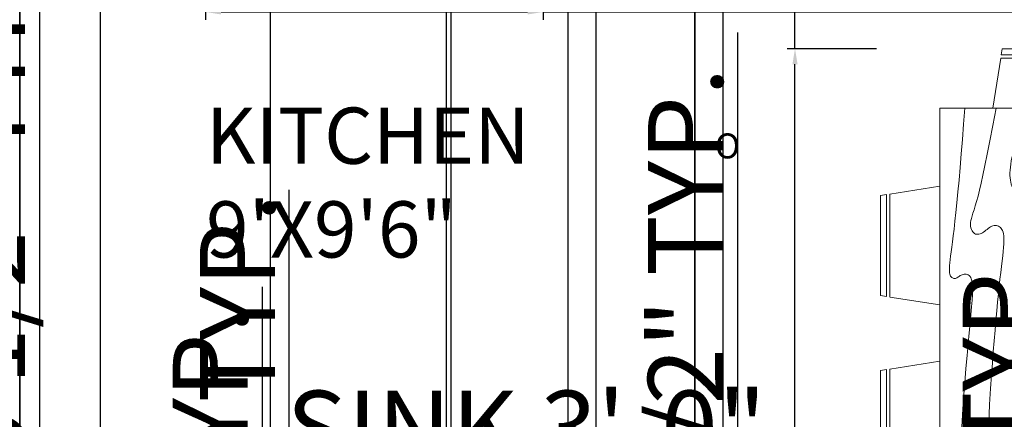
# Model space of a CAD drawing. Units: inches. Extents: x 2691 to 3133, y 1294 to 1993.
# Tile 5 of 7: x 2777 to 2935, y 1798 to 1862. Entities that reach past the tile are written whole.
import ezdxf

# ---------------------------------------------------------------- set-up
doc = ezdxf.new("R2010")
doc.units = ezdxf.units.IN
for name, color, linetype, lineweight in [('A-ANNO-DIMS', 2, 'Continuous', 18), ('A-ANNO-TEXT', 7, 'Continuous', 18), ('A-AREA-IDEN', 7, 'Continuous', 25), ('A-FURN', 8, 'Continuous', 18), ('A-WALL', 7, 'Continuous', 35)]:
    doc.layers.add(name, color=color, linetype=linetype, lineweight=lineweight)
doc.styles.get("Standard").update_dxf_attribs({"font": 'arial.ttf'})
doc.dimstyles.new('ISO-25', dxfattribs={"dimtxt": 12, "dimasz": 2.5, "dimexe": 1.25, "dimexo": 0.625, "dimtad": 1, "dimdec": 1, "dimlunit": 3, "dimtxsty": 'Standard', "dimcen": 2.5, "dimadec": 0, "dimazin": 0, "dimtfac": 1, "dimtdec": 1, "dimtmove": 0, "dimatfit": 3, "dimfxl": 1, "dimarcsym": 0})

# ---------------------------------------------------------------- blocks, each defined once
blk = doc.blocks.new('Dining Set - 36 x 72 in.')
for p, q in [((-22, 27.5), (-22.1562, 26.50042)), ((-22, 27.5), (-6, 27.5)), ((-5.8437, 26.49966), (-6, 27.5)), ((6, 27.5), (5.8438, 26.50042)), ((6, 27.5), (22, 27.5)), ((22.1563, 26.49966), (22, 27.5)), ((-22.2343, 26.00059), (-23.4847, 17.99762)), ((-22.2304, 26), (-5.7608, 26)), ((-5.8416, 26.5), (-22.1534, 26.5)), ((-4.5152, 17.99762), (-5.7655, 25.99926)), ((5.7657, 26.00059), (4.5153, 17.99762)), ((5.7696, 26), (22.2392, 26)), ((22.1584, 26.5), (5.8466, 26.5)), ((23.4848, 17.99762), (22.2345, 25.99926)), ((36, 18), (-36, 18)), ((-36, 18), (-36, -18)), ((36, -18), (36, 18)), ((-44.0006, 8.23428), (-35.9976, 9.48474)), ((44.0006, 8.23428), (35.9976, 9.48474)), ((-45.5, 8), (-44.5004, 8.15617)), ((-45.5, 8), (-45.5, -8)), ((-44.5, -8.15843), (-44.5, 8.15338)), ((-44, 8.23041), (-44, -8.23915)), ((44, 8.23041), (44, -8.23915)), ((44.5, -8.15843), (44.5, 8.15338)), ((45.5, 8), (44.5005, 8.15617)), ((45.5, 8), (45.5, -8)), ((-44.4997, -8.15631), (-45.5, -8)), ((-35.9976, -9.48476), (-43.9993, -8.2345)), ((35.9976, -9.48476), (43.9993, -8.2345)), ((44.4997, -8.15631), (45.5, -8)), ((-36, -18), (36, -18)), ((-22.2343, -26.0006), (-23.4847, -17.99762)), ((-4.5152, -17.99762), (-5.7655, -25.99928)), ((5.7657, -26.0006), (4.5153, -17.99762)), ((23.4848, -17.99762), (22.2345, -25.99928)), ((-22.2304, -26), (-5.7608, -26)), ((-22, -27.5), (-22.1562, -26.50044)), ((-5.8416, -26.5), (-22.1534, -26.5)), ((-5.8437, -26.49967), (-6, -27.5)), ((5.7696, -26), (22.2392, -26)), ((6, -27.5), (5.8438, -26.50044)), ((22.1584, -26.5), (5.8466, -26.5)), ((22.1563, -26.49967), (22, -27.5)), ((-22, -27.5), (-6, -27.5)), ((6, -27.5), (22, -27.5))]:
    blk.add_line(p, q)
for points in [[(-36, 15), (-31.1772, 14.97754), (-26.8079, 14.91406), (-22.8538, 14.81543), (-19.276, 14.6875), (-16.0362, 14.53613), (-13.0957, 14.36718), (-10.4159, 14.18652), (-7.9583, 14), (-5.6904, 13.81315), (-3.6035, 13.63021), (-1.6954, 13.45508), (0.0365, 13.29166), (1.5945, 13.14388), (2.9811, 13.01562), (4.1988, 12.9108), (5.25, 12.83333), (6.1393, 12.78613), (6.8802, 12.76823), (7.4883, 12.77767), (7.9792, 12.8125), (8.3685, 12.87077), (8.6719, 12.95052), (8.9049, 13.0498), (9.0833, 13.16666), (9.2205, 13.29899), (9.3216, 13.44401), (9.3895, 13.59879), (9.4271, 13.76041), (9.4373, 13.92594), (9.4232, 14.09245), (9.3875, 14.257), (9.3333, 14.41666), (9.2638, 14.56917), (9.1836, 14.71484), (9.0975, 14.85465), (9.0104, 14.98958), (8.9272, 15.1206), (8.8529, 15.2487), (8.7922, 15.37483), (8.75, 15.5), (8.7305, 15.62467), (8.7344, 15.74739), (8.7617, 15.86621), (8.8125, 15.97916), (8.8867, 16.08431), (8.9844, 16.17968), (9.1055, 16.26334), (9.25, 16.33333), (9.4189, 16.38802), (9.6172, 16.42708), (9.8506, 16.45052), (10.125, 16.45833), (10.4463, 16.45052), (10.8203, 16.42708), (11.2529, 16.38802), (11.75, 16.33333), (12.3184, 16.26318), (12.9694, 16.17838), (13.7151, 16.07991), (14.5677, 15.96875), (15.5395, 15.84586), (16.6426, 15.71224), (17.8893, 15.56884), (19.2917, 15.41666), (20.859, 15.25667), (22.5879, 15.08984), (24.4721, 14.91715), (26.5052, 14.73958), (28.6809, 14.5581), (30.9929, 14.3737), (33.4347, 14.18733), (36, 14)], [(-36, 10), (-28.9766, 10.14274), (-23.1725, 10.20442), (-18.4241, 10.19775), (-14.5677, 10.13541), (-11.4399, 10.03011), (-8.877, 9.89453), (-6.7154, 9.74137), (-4.7917, 9.58333), (-2.9698, 9.43082), (-1.2246, 9.28515), (0.4415, 9.14534), (2.026, 9.01041), (3.5266, 8.87939), (4.9408, 8.7513), (6.266, 8.62516), (7.5, 8.5), (8.6411, 8.37549), (9.6914, 8.2539), (10.6538, 8.13818), (11.5312, 8.03125), (12.3267, 7.93603), (13.043, 7.85547), (13.6831, 7.79248), (14.25, 7.75), (14.7471, 7.7303), (15.1797, 7.73307), (15.5537, 7.75732), (15.875, 7.80208), (16.1494, 7.86637), (16.3828, 7.94922), (16.5811, 8.04964), (16.75, 8.16666), (16.8944, 8.29915), (17.0143, 8.44531), (17.1089, 8.60319), (17.1771, 8.77083), (17.218, 8.94629), (17.2305, 9.1276), (17.2137, 9.31282), (17.1667, 9.5), (17.0895, 9.6875), (16.987, 9.875), (16.8649, 10.0625), (16.7292, 10.25), (16.5856, 10.4375), (16.4401, 10.625), (16.2985, 10.8125), (16.1667, 11), (16.05, 11.18733), (15.9518, 11.3737), (15.8752, 11.5581), (15.8229, 11.73958), (15.798, 11.91715), (15.8034, 12.08984), (15.842, 12.25667), (15.9167, 12.41666), (16.0295, 12.56836), (16.1784, 12.70833), (16.3605, 12.83268), (16.5729, 12.9375), (16.8127, 13.01888), (17.0768, 13.07291), (17.3625, 13.0957), (17.6667, 13.08333), (17.9894, 13.03312), (18.3418, 12.94726), (18.7382, 12.82918), (19.1927, 12.68229), (19.7195, 12.51001), (20.3327, 12.31575), (21.0465, 12.10294), (21.875, 11.875), (22.8357, 11.63354), (23.959, 11.37304), (25.2786, 11.08618), (26.8282, 10.76562), (28.6414, 10.40405), (30.752, 9.99414), (33.1936, 9.52856), (36, 9)], [(-36, 5.5), (-30.7157, 5.3348), (-26.069, 5.20963), (-21.9946, 5.11767), (-18.4271, 5.05208), (-15.3009, 5.00602), (-12.5508, 4.97265), (-10.1112, 4.94515), (-7.9167, 4.91666), (-5.909, 4.88167), (-4.0586, 4.83984), (-2.3429, 4.79215), (-0.7396, 4.73958), (0.7739, 4.6831), (2.22, 4.6237), (3.6213, 4.56233), (5, 4.5), (6.373, 4.43782), (7.7344, 4.3776), (9.0723, 4.32129), (10.375, 4.27083), (11.6309, 4.22819), (12.8281, 4.19531), (13.9551, 4.17415), (15, 4.16666), (15.954, 4.17448), (16.819, 4.19791), (17.6001, 4.23698), (18.3021, 4.29166), (18.9299, 4.36198), (19.4883, 4.44791), (19.9823, 4.54948), (20.4167, 4.66666), (20.7969, 4.79899), (21.1302, 4.94401), (21.4245, 5.09879), (21.6875, 5.26041), (21.9271, 5.42594), (22.1511, 5.59245), (22.3672, 5.757), (22.5834, 5.91666), (22.8065, 6.06868), (23.0404, 6.21093), (23.2879, 6.34147), (23.5521, 6.45833), (23.8358, 6.55957), (24.142, 6.64323), (24.4735, 6.70735), (24.8334, 6.75), (25.2235, 6.76969), (25.642, 6.76692), (26.0858, 6.74267), (26.5521, 6.69791), (27.0379, 6.63362), (27.5404, 6.55078), (28.0565, 6.45036), (28.5834, 6.33333), (29.1242, 6.19987), (29.7071, 6.04687), (30.3661, 5.87044), (31.1354, 5.66666), (32.0493, 5.43164), (33.142, 5.16146), (34.4475, 4.85221), (36, 4.5)], [(-36, -1), (-30.7915, -0.6591), (-26.0195, -0.38216), (-21.6519, -0.16284), (-17.6563, 0.00521), (-14.0005, 0.12833), (-10.6523, 0.21289), (-7.5796, 0.26522), (-4.75, 0.29166), (-2.134, 0.29793), (0.2878, 0.28711), (2.5317, 0.26163), (4.6146, 0.22396), (6.5529, 0.17651), (8.3633, 0.12174), (10.0623, 0.06209), (11.6667, 0), (13.1899, -0.06201), (14.6341, -0.1211), (15.9982, -0.17432), (17.2813, -0.21875), (18.4823, -0.25147), (19.6003, -0.26953), (20.6343, -0.27002), (21.5834, -0.25), (22.4481, -0.20768), (23.2357, -0.14584), (23.9549, -0.06836), (24.6146, 0.02083), (25.2235, 0.11784), (25.7904, 0.21875), (26.3241, 0.31966), (26.8334, 0.41666), (27.3265, 0.50618), (27.8099, 0.58593), (28.2894, 0.65397), (28.7709, 0.70833), (29.2601, 0.74707), (29.763, 0.76823), (30.2855, 0.76985), (30.8334, 0.75), (31.4088, 0.70784), (31.9994, 0.64713), (32.589, 0.57275), (33.1615, 0.48958), (33.7008, 0.4025), (34.1908, 0.3164), (34.6153, 0.23616), (34.9584, 0.16666), (35.2099, 0.11165), (35.3848, 0.07031), (35.504, 0.04069), (35.5886, 0.02083), (35.6594, 0.00879), (35.7377, 0.0026), (35.8442, 0.00032), (36, 0)], [(-36, -6.5), (-27.1843, -6.31267), (-20.084, -6.1263), (-14.469, -5.9419), (-10.1094, -5.76042), (-6.7752, -5.58285), (-4.2363, -5.41016), (-2.2629, -5.24333), (-0.625, -5.08334), (0.8708, -4.93099), (2.2715, -4.78646), (3.5872, -4.64974), (4.8281, -4.52084), (6.0046, -4.39974), (7.127, -4.28646), (8.2053, -4.18099), (9.25, -4.08334), (10.2705, -3.99382), (11.2734, -3.91407), (12.2647, -3.84603), (13.25, -3.79167), (14.2354, -3.75293), (15.2266, -3.73177), (16.2295, -3.73015), (17.25, -3.75), (18.2912, -3.79248), (19.3451, -3.85547), (20.4009, -3.93604), (21.4479, -4.03125), (22.4754, -4.13819), (23.4727, -4.25391), (24.4289, -4.37549), (25.3334, -4.5), (26.1785, -4.62492), (26.9694, -4.74935), (27.7145, -4.87281), (28.4219, -4.99479), (29.1, -5.11483), (29.7572, -5.23242), (30.4016, -5.34709), (31.0417, -5.45834), (31.6837, -5.56437), (32.3262, -5.65821), (32.9658, -5.73153), (33.599, -5.77604), (34.2224, -5.78345), (34.8327, -5.74545), (35.4264, -5.65373), (36, -5.5)], [(-36, -10), (-26.4022, -9.81299), (-18.4675, -9.62891), (-11.9839, -9.45069), (-6.7396, -9.28125), (-2.5226, -9.12354), (0.8789, -8.98047), (3.6769, -8.85498), (6.0833, -8.75), (8.2767, -8.66765), (10.3021, -8.60677), (12.1712, -8.56543), (13.8958, -8.54167), (15.4876, -8.53353), (16.9583, -8.53907), (18.3197, -8.55632), (19.5834, -8.58334), (20.7616, -8.61841), (21.8685, -8.66081), (22.9188, -8.71004), (23.9271, -8.76563), (24.9081, -8.82707), (25.8763, -8.89388), (26.8465, -8.96558), (27.8334, -9.04167), (28.8474, -9.12118), (29.8828, -9.20117), (30.93, -9.27824), (31.9792, -9.34896), (33.0205, -9.40991), (34.0443, -9.45768), (35.0407, -9.48885), (36, -9.5)], [(-36, -14.5), (-30.0881, -14.33513), (-25.0332, -14.21224), (-20.7312, -14.12647), (-17.0781, -14.07292), (-13.97, -14.04671), (-11.3027, -14.04297), (-8.9724, -14.05681), (-6.875, -14.08334), (-4.9224, -14.11833), (-3.0905, -14.16016), (-1.3709, -14.20785), (0.2448, -14.26042), (1.7647, -14.3169), (3.1973, -14.3763), (4.5507, -14.43767), (5.8333, -14.5), (7.0554, -14.5621), (8.235, -14.62175), (9.3922, -14.67652), (10.5469, -14.72396), (11.7192, -14.76164), (12.929, -14.78711), (14.1965, -14.79794), (15.5417, -14.79167), (16.9933, -14.76424), (18.6152, -14.70508), (20.4804, -14.60197), (22.6615, -14.44271), (25.2312, -14.21509), (28.2624, -13.9069), (31.8277, -13.50594), (36, -13)]]:
    blk.add_lwpolyline(points)
blk = doc.blocks.new('*D14')
at = {"layer": 'A-ANNO-DIMS', "color": 0, "lineweight": -2, "transparency": 16777216}
for p, q in [((2806.97, 1870.43), (2806.97, 1861.7)), ((2860.97, 1870.43), (2860.97, 1861.7)), ((2809.47, 1862.95), (2858.47, 1862.95)), ((2860.97, 1862.95), (3015.92, 1862.95))]:
    blk.add_line(p, q, dxfattribs=at)
at = {"layer": 'A-ANNO-DIMS', "color": 0, "transparency": 16777216}
for points in [[(2809.47, 1863.37), (2809.47, 1862.54), (2806.97, 1862.95)], [(2858.47, 1863.37), (2858.47, 1862.54), (2860.97, 1862.95)]]:
    blk.add_solid(points, dxfattribs=at)
at = {"layer": 'Defpoints', "color": 0, "transparency": 16777216}
for p in [(2806.97, 1871.05), (2860.97, 1871.05), (2860.97, 1862.95)]:
    blk.add_point(p, dxfattribs=at)
at = {"layer": 'A-ANNO-DIMS', "color": 0, "transparency": 16777216, "insert": (2939.69, 1869.78), "char_height": 12, "attachment_point": 5}
blk.add_mtext('GLAZING 4\'-6" TYP.', dxfattribs=at)
blk = doc.blocks.new('*D18')
at = {"layer": 'A-ANNO-DIMS', "color": 0, "lineweight": -2, "transparency": 16777216}
for p, q in [((2780.49, 1693.45), (2780.49, 1876.36)), ((2777.87, 1693.45), (2781.74, 1693.45)), ((2780.49, 1674.35), (2780.49, 1690.95)), ((2777.87, 1671.85), (2781.74, 1671.85))]:
    blk.add_line(p, q, dxfattribs=at)
at = {"layer": 'A-ANNO-DIMS', "color": 0, "transparency": 16777216}
for points in [[(2780.07, 1690.95), (2780.91, 1690.95), (2780.49, 1693.45)], [(2780.07, 1674.35), (2780.91, 1674.35), (2780.49, 1671.85)]]:
    blk.add_solid(points, dxfattribs=at)
at = {"layer": 'Defpoints', "color": 0, "transparency": 16777216}
for p in [(2777.25, 1693.45), (2780.49, 1693.45), (2777.25, 1671.85)]:
    blk.add_point(p, dxfattribs=at)
at = {"layer": 'A-ANNO-DIMS', "color": 0, "transparency": 16777216, "insert": (2773.66, 1786.16), "char_height": 12, "attachment_point": 5, "rotation": 90}
blk.add_mtext('GLAZING 1\'-9 1/2" TYP.', dxfattribs=at)
blk = doc.blocks.new('*D20')
at = {"layer": 'A-ANNO-DIMS', "color": 0, "lineweight": -2, "transparency": 16777216}
for p, q in [((2942.46, 1702.1), (2942.46, 1829.23)), ((2930.49, 1702.1), (2943.71, 1702.1)), ((2942.46, 1620.6), (2942.46, 1699.6)), ((2930.49, 1618.1), (2943.71, 1618.1))]:
    blk.add_line(p, q, dxfattribs=at)
at = {"layer": 'A-ANNO-DIMS', "color": 0, "transparency": 16777216}
for points in [[(2942.05, 1699.6), (2942.88, 1699.6), (2942.46, 1702.1)], [(2942.05, 1620.6), (2942.88, 1620.6), (2942.46, 1618.1)]]:
    blk.add_solid(points, dxfattribs=at)
at = {"layer": 'Defpoints', "color": 0, "transparency": 16777216}
for p in [(2929.86, 1702.1), (2942.46, 1702.1), (2929.86, 1618.1)]:
    blk.add_point(p, dxfattribs=at)
at = {"layer": 'A-ANNO-DIMS', "color": 0, "transparency": 16777216, "insert": (2935.63, 1766.91), "char_height": 12, "attachment_point": 5, "rotation": 90}
blk.add_mtext('SOFA 7\'-0" TYP.', dxfattribs=at)
blk = doc.blocks.new('*D22')
at = {"layer": 'A-ANNO-DIMS', "color": 0, "lineweight": -2, "transparency": 16777216}
for p, q in [((2816.11, 1708.98), (2816.11, 1818.95)), ((2811.78, 1708.98), (2817.36, 1708.98)), ((2816.11, 1678.43), (2816.11, 1706.48)), ((2811.78, 1675.93), (2817.36, 1675.93))]:
    blk.add_line(p, q, dxfattribs=at)
at = {"layer": 'A-ANNO-DIMS', "color": 0, "transparency": 16777216}
for points in [[(2815.69, 1706.48), (2816.52, 1706.48), (2816.11, 1708.98)], [(2815.69, 1678.43), (2816.52, 1678.43), (2816.11, 1675.93)]]:
    blk.add_solid(points, dxfattribs=at)
at = {"layer": 'Defpoints', "color": 0, "transparency": 16777216}
for p in [(2811.15, 1708.98), (2816.11, 1708.98), (2811.15, 1675.93)]:
    blk.add_point(p, dxfattribs=at)
at = {"layer": 'A-ANNO-DIMS', "color": 0, "transparency": 16777216, "insert": (2809.28, 1765.22), "char_height": 12, "attachment_point": 5, "rotation": 90}
blk.add_mtext('WC 2\'-9" TYP.', dxfattribs=at)
blk = doc.blocks.new('*D24')
at = {"layer": 'A-ANNO-DIMS', "color": 0, "lineweight": -2, "transparency": 16777216}
for p, q in [((2823.75, 1755.69), (2823.75, 1759.69)), ((2846.25, 1755.69), (2846.25, 1759.69)), ((2826.25, 1758.44), (2843.75, 1758.44)), ((2846.25, 1758.44), (3032.5, 1758.44))]:
    blk.add_line(p, q, dxfattribs=at)
at = {"layer": 'A-ANNO-DIMS', "color": 0, "transparency": 16777216}
for points in [[(2826.25, 1758.86), (2826.25, 1758.02), (2823.75, 1758.44)], [(2843.75, 1758.86), (2843.75, 1758.02), (2846.25, 1758.44)]]:
    blk.add_solid(points, dxfattribs=at)
at = {"layer": 'Defpoints', "color": 0, "transparency": 16777216}
for p in [(2846.25, 1758.44), (2823.75, 1755.06), (2846.25, 1755.06)]:
    blk.add_point(p, dxfattribs=at)
at = {"layer": 'A-ANNO-DIMS', "color": 0, "transparency": 16777216, "insert": (2940.63, 1765.27), "char_height": 12, "attachment_point": 5}
blk.add_mtext('D1 LEAF 1\'-10 1/2" TYP.', dxfattribs=at)
blk = doc.blocks.new('*D25')
at = {"layer": 'A-ANNO-DIMS', "color": 0, "lineweight": -2, "transparency": 16777216}
for p, q in [((2820.37, 1757.56), (2820.37, 1834.46)), ((2823.12, 1755.06), (2819.12, 1755.06)), ((2820.37, 1754.06), (2820.37, 1755.06)), ((2823.12, 1754.06), (2819.12, 1754.06)), ((2820.37, 1751.56), (2820.37, 1749.06))]:
    blk.add_line(p, q, dxfattribs=at)
at = {"layer": 'A-ANNO-DIMS', "color": 0, "transparency": 16777216}
for points in [[(2819.96, 1757.56), (2820.79, 1757.56), (2820.37, 1755.06)], [(2819.96, 1751.56), (2820.79, 1751.56), (2820.37, 1754.06)]]:
    blk.add_solid(points, dxfattribs=at)
at = {"layer": 'Defpoints', "color": 0, "transparency": 16777216}
for p in [(2820.37, 1755.06), (2823.75, 1755.06), (2823.75, 1754.06)]:
    blk.add_point(p, dxfattribs=at)
at = {"layer": 'A-ANNO-DIMS', "color": 0, "transparency": 16777216, "insert": (2813.62, 1797.26), "char_height": 12, "attachment_point": 5, "rotation": 90}
blk.add_mtext('0\'-1" TYP.', dxfattribs=at)
blk = doc.blocks.new('*D26')
at = {"layer": 'A-ANNO-DIMS', "color": 0, "lineweight": -2, "transparency": 16777216}
for p, q in [((2892.12, 1644.55), (2892.12, 1859.67)), ((2889.37, 1644.55), (2893.37, 1644.55)), ((2892.12, 1624.55), (2892.12, 1642.05)), ((2889.37, 1622.05), (2893.37, 1622.05))]:
    blk.add_line(p, q, dxfattribs=at)
at = {"layer": 'A-ANNO-DIMS', "color": 0, "transparency": 16777216}
for points in [[(2891.71, 1642.05), (2892.54, 1642.05), (2892.12, 1644.55)], [(2891.71, 1624.55), (2892.54, 1624.55), (2892.12, 1622.05)]]:
    blk.add_solid(points, dxfattribs=at)
at = {"layer": 'Defpoints', "color": 0, "transparency": 16777216}
for p in [(2888.75, 1644.55), (2892.12, 1644.55), (2888.75, 1622.05)]:
    blk.add_point(p, dxfattribs=at)
at = {"layer": 'A-ANNO-DIMS', "color": 0, "transparency": 16777216, "insert": (2885.29, 1753.36), "char_height": 12, "attachment_point": 5, "rotation": 90}
blk.add_mtext('DOOR LEAF 1\'-10 1/2" TYP.', dxfattribs=at)
blk = doc.blocks.new('*D30')
at = {"layer": 'A-ANNO-DIMS', "color": 0, "lineweight": -2, "transparency": 16777216}
for p, q in [((2901.25, 1857.07), (2901.25, 1992.71)), ((2914.28, 1857.07), (2900, 1857.07)), ((2901.25, 1768.57), (2901.25, 1854.57)), ((2914.28, 1766.07), (2900, 1766.07))]:
    blk.add_line(p, q, dxfattribs=at)
at = {"layer": 'A-ANNO-DIMS', "color": 0, "transparency": 16777216}
for points in [[(2900.84, 1854.57), (2901.67, 1854.57), (2901.25, 1857.07)], [(2900.84, 1768.57), (2901.67, 1768.57), (2901.25, 1766.07)]]:
    blk.add_solid(points, dxfattribs=at)
at = {"layer": 'Defpoints', "color": 0, "transparency": 16777216}
for p in [(2901.25, 1857.07), (2914.9, 1857.07), (2914.9, 1766.07)]:
    blk.add_point(p, dxfattribs=at)
at = {"layer": 'A-ANNO-DIMS', "color": 0, "transparency": 16777216, "insert": (2894.42, 1926.14), "char_height": 12, "attachment_point": 5, "rotation": 90}
blk.add_mtext('DINING SET 7\'-7"', dxfattribs=at)
blk = doc.blocks.new('*D36')
at = {"layer": 'A-ANNO-DIMS', "color": 0, "lineweight": -2, "transparency": 16777216}
for p, q in [((2781.34, 1783.18), (2781.34, 1789.2)), ((2817.34, 1783.18), (2817.34, 1789.2)), ((2783.84, 1787.95), (2814.84, 1787.95)), ((2817.34, 1787.95), (2896.72, 1787.95))]:
    blk.add_line(p, q, dxfattribs=at)
at = {"layer": 'A-ANNO-DIMS', "color": 0, "transparency": 16777216}
for points in [[(2783.84, 1788.37), (2783.84, 1787.54), (2781.34, 1787.95)], [(2814.84, 1788.37), (2814.84, 1787.54), (2817.34, 1787.95)]]:
    blk.add_solid(points, dxfattribs=at)
at = {"layer": 'Defpoints', "color": 0, "transparency": 16777216}
for p in [(2817.34, 1787.95), (2781.34, 1782.55), (2817.34, 1782.55)]:
    blk.add_point(p, dxfattribs=at)
at = {"layer": 'A-ANNO-DIMS', "color": 0, "transparency": 16777216, "insert": (2858.28, 1794.79), "char_height": 12, "attachment_point": 5}
blk.add_mtext('SINK 3\'-0"', dxfattribs=at)
blk = doc.blocks.new('*D54')
at = {"layer": 'A-ANNO-DIMS', "color": 0, "lineweight": -2, "transparency": 16777216}
for p, q in [((2846.25, 1645.18), (2846.25, 1905.15)), ((2848.75, 1903.9), (2866.94, 1903.9)), ((2869.44, 1645.18), (2869.44, 1905.15)), ((2869.44, 1903.9), (2913.28, 1903.9))]:
    blk.add_line(p, q, dxfattribs=at)
at = {"layer": 'A-ANNO-DIMS', "color": 0, "transparency": 16777216}
for points in [[(2848.75, 1904.32), (2848.75, 1903.49), (2846.25, 1903.9)], [(2866.94, 1904.32), (2866.94, 1903.49), (2869.44, 1903.9)]]:
    blk.add_solid(points, dxfattribs=at)
at = {"layer": 'Defpoints', "color": 0, "transparency": 16777216}
for p in [(2869.44, 1903.9), (2846.25, 1644.55), (2869.44, 1644.55)]:
    blk.add_point(p, dxfattribs=at)
at = {"layer": 'A-ANNO-DIMS', "color": 0, "transparency": 16777216, "insert": (2892.61, 1910.55), "char_height": 12, "attachment_point": 5}
blk.add_mtext('1\'-11"', dxfattribs=at)
blk = doc.blocks.new('*D57')
at = {"layer": 'A-ANNO-DIMS', "color": 0, "lineweight": -2, "transparency": 16777216}
for p, q in [((2777.25, 1709.68), (2777.25, 1905.15)), ((2779.75, 1903.9), (2787.65, 1903.9)), ((2790.15, 1709.61), (2790.15, 1905.15)), ((2790.15, 1903.9), (2824.67, 1903.9))]:
    blk.add_line(p, q, dxfattribs=at)
at = {"layer": 'A-ANNO-DIMS', "color": 0, "transparency": 16777216}
for points in [[(2779.75, 1904.32), (2779.75, 1903.49), (2777.25, 1903.9)], [(2787.65, 1904.32), (2787.65, 1903.49), (2790.15, 1903.9)]]:
    blk.add_solid(points, dxfattribs=at)
at = {"layer": 'Defpoints', "color": 0, "transparency": 16777216}
for p in [(2790.15, 1903.9), (2777.25, 1709.05), (2790.15, 1708.98)]:
    blk.add_point(p, dxfattribs=at)
at = {"layer": 'A-ANNO-DIMS', "color": 0, "transparency": 16777216, "insert": (2808.66, 1910.55), "char_height": 12, "attachment_point": 5}
blk.add_mtext('1\'-1"', dxfattribs=at)
blk = doc.blocks.new('*D60')
at = {"layer": 'A-ANNO-DIMS', "color": 0, "lineweight": -2, "transparency": 16777216}
for p, q in [((2817.34, 1781.68), (2817.34, 1905.15)), ((2819.84, 1903.9), (2843.03, 1903.9)), ((2845.53, 1786.1), (2845.53, 1905.15)), ((2845.53, 1903.9), (2881.38, 1903.9))]:
    blk.add_line(p, q, dxfattribs=at)
at = {"layer": 'A-ANNO-DIMS', "color": 0, "transparency": 16777216}
for points in [[(2819.84, 1904.32), (2819.84, 1903.49), (2817.34, 1903.9)], [(2843.03, 1904.32), (2843.03, 1903.49), (2845.53, 1903.9)]]:
    blk.add_solid(points, dxfattribs=at)
at = {"layer": 'Defpoints', "color": 0, "transparency": 16777216}
for p in [(2845.53, 1903.9), (2845.53, 1785.48), (2817.34, 1781.05)]:
    blk.add_point(p, dxfattribs=at)
at = {"layer": 'A-ANNO-DIMS', "color": 0, "transparency": 16777216, "insert": (2864.71, 1910.55), "char_height": 12, "attachment_point": 5}
blk.add_mtext('2\'-4"', dxfattribs=at)
blk = doc.blocks.new('*D61')
at = {"layer": 'A-ANNO-DIMS', "color": 0, "lineweight": -2, "transparency": 16777216}
for p, q in [((2864.96, 1433.88), (2864.96, 1905.15)), ((2867.46, 1903.9), (2887.25, 1903.9)), ((2889.75, 1433.68), (2889.75, 1905.15)), ((2889.75, 1903.9), (2925.6, 1903.9))]:
    blk.add_line(p, q, dxfattribs=at)
at = {"layer": 'A-ANNO-DIMS', "color": 0, "transparency": 16777216}
for points in [[(2867.46, 1904.32), (2867.46, 1903.49), (2864.96, 1903.9)], [(2887.25, 1904.32), (2887.25, 1903.49), (2889.75, 1903.9)]]:
    blk.add_solid(points, dxfattribs=at)
at = {"layer": 'Defpoints', "color": 0, "transparency": 16777216}
for p in [(2889.75, 1903.9), (2864.96, 1433.26), (2889.75, 1433.05)]:
    blk.add_point(p, dxfattribs=at)
at = {"layer": 'A-ANNO-DIMS', "color": 0, "transparency": 16777216, "insert": (2908.93, 1910.55), "char_height": 12, "attachment_point": 5}
blk.add_mtext('2\'-1"', dxfattribs=at)

msp = doc.modelspace()

# ---------------------------------------------------------------- linework, layer by layer
at = {"layer": 'A-WALL'}
for p, q in [((2777.25, 1871.05), (2777.25, 1761.55)), ((2885.25, 1796.11), (2885.25, 1871.05))]:
    msp.add_line(p, q, dxfattribs=at)

# ---------------------------------------------------------------- block references
at = {"layer": 'A-FURN', "rotation": 90}
msp.add_blockref('Dining Set - 36 x 72 in.', (2942.4, 1811.57), dxfattribs=at)

# ---------------------------------------------------------------- texts
at = {"layer": 'A-ANNO-TEXT', "insert": (2888.43, 1843.51), "char_height": 4, "attachment_point": 1}
msp.add_mtext_dynamic_manual_height_columns('O', width=0.1038, gutter_width=12.5, heights=[0], dxfattribs=at)
at = {"layer": 'A-AREA-IDEN', "insert": (2807.05, 1847.65), "char_height": 9, "attachment_point": 1}
msp.add_mtext('KITCHEN\\P9\'X9\'6"', dxfattribs=at)

# ---------------------------------------------------------------- dimensions: what is measured, and where the dimension line sits
at = {"layer": 'A-ANNO-DIMS'}
for base, p1, p2, text, picture, middle in [((2901.25, 1857.07), (2914.9, 1766.07), (2914.9, 1857.07), 'DINING SET <>', '*D30', (2894.42, 1926.14)), ((2780.49, 1693.45), (2777.25, 1671.85), (2777.25, 1693.45), 'GLAZING <> TYP.', '*D18', (2773.66, 1786.16)), ((2892.12, 1644.55), (2888.75, 1622.05), (2888.75, 1644.55), 'DOOR LEAF <> TYP.', '*D26', (2885.29, 1753.36)), ((2820.37, 1755.06), (2823.75, 1754.06), (2823.75, 1755.06), '<> TYP.', '*D25', (2813.62, 1797.26)), ((2942.46, 1702.1), (2929.86, 1618.1), (2929.86, 1702.1), 'SOFA <> TYP.', '*D20', (2935.63, 1766.91)), ((2816.1072, 1708.9801), (2811.1502, 1675.9339), (2811.1502, 1708.9801), 'WC <> TYP.', '*D22', (2809.2775, 1765.217))]:
    dim = msp.add_linear_dim(base=base, p1=p1, p2=p2, angle=90, text=text, dimstyle='ISO-25', override={"dimdec": 1, "dimlfac": 1, "dimrnd": 0, "dimzin": 1, "dimdsep": 46, "dimlunit": 4, "dimfrac": 2}, dxfattribs=at)
    dim.commit()
    dim.dimension.update_dxf_attribs({"geometry": picture, "text_midpoint": middle})
for base, p1, p2, picture, middle in [((2790.15, 1903.9), (2777.25, 1709.05), (2790.15, 1708.98), '*D57', (2808.66, 1910.55)), ((2845.53, 1903.9), (2817.34, 1781.05), (2845.53, 1785.48), '*D60', (2864.71, 1910.55)), ((2869.44, 1903.9), (2846.25, 1644.55), (2869.44, 1644.55), '*D54', (2892.61, 1910.55)), ((2889.75, 1903.9), (2864.96, 1433.26), (2889.75, 1433.05), '*D61', (2908.93, 1910.55))]:
    dim = msp.add_linear_dim(base=base, p1=p1, p2=p2, dimstyle='ISO-25', override={"dimdec": 1, "dimlfac": 1, "dimrnd": 0, "dimzin": 1, "dimdsep": 46, "dimlunit": 4, "dimfrac": 2}, dxfattribs=at)
    dim.commit()
    dim.dimension.update_dxf_attribs({"geometry": picture, "text_midpoint": middle})
for base, p1, p2, text, picture, middle in [((2860.97, 1862.95), (2806.97, 1871.05), (2860.97, 1871.05), 'GLAZING <> TYP.', '*D14', (2939.69, 1869.78)), ((2817.34, 1787.95), (2781.34, 1782.55), (2817.34, 1782.55), 'SINK <>', '*D36', (2858.28, 1794.79)), ((2846.25, 1758.44), (2823.75, 1755.06), (2846.25, 1755.06), 'D1 LEAF <> TYP.', '*D24', (2940.63, 1765.27))]:
    dim = msp.add_linear_dim(base=base, p1=p1, p2=p2, text=text, dimstyle='ISO-25', override={"dimdec": 1, "dimlfac": 1, "dimrnd": 0, "dimzin": 1, "dimdsep": 46, "dimlunit": 4, "dimfrac": 2}, dxfattribs=at)
    dim.commit()
    dim.dimension.update_dxf_attribs({"geometry": picture, "text_midpoint": middle})

doc.saveas('drawing.dxf')
